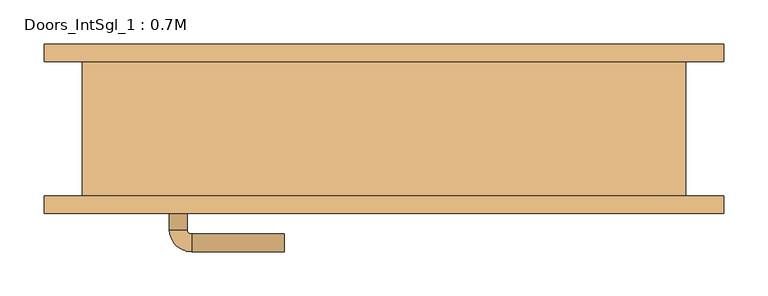
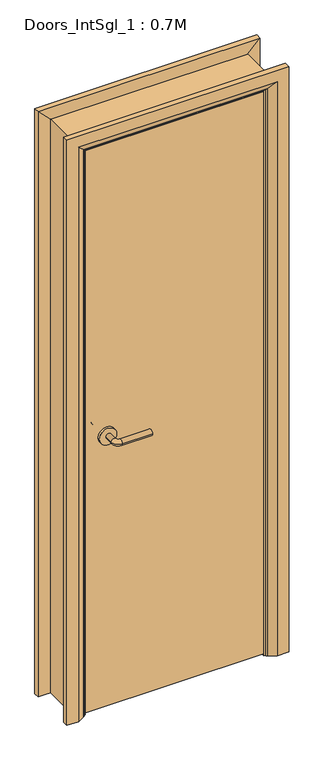
"""IFC4 building model written with IfcOpenShell, lengths in millimetres: door geometry, Doors_IntSgl_1 : 0.7M."""

from ifc_helpers import new_model, si_unit, point, frame, frame_2d, origin, place, context, project, spatial, polyline, circle_curve, ellipse_curve, trimmed, segment, composite_curve, outline, extrude, faceted_brep, source, transform, mapped, element, save
from ifc_brep_helpers import plane_surface, cylinder_surface, revolved_surface, advanced_brep


def doors_intsgl_1_0_7m_20e7f540(model_context):
    return source(origin(), model_context, "Body", "SolidModel", [
        advanced_brep(
        [(-243.0, -30.2, 1000.0), (-223.0, -30.2, 1000.0), (-243.0, -0.2, 1000.0), (-223.0, -0.2, 1000.0), (-218.0, 4.8, 1000.0), (-218.0, 24.8, 1000.0), (-113.0, 24.8, 1000.0), (-113.0, 4.8, 1000.0)],
        [
            (0, 1, circle_curve(frame((-233.0, -30.2, 1000.0), z_axis=(0.0, -1.0, 0.0), x_axis=(1.0, 0.0, 0.0)), 10.0)),
            (1, 0, circle_curve(frame((-233.0, -30.2, 1000.0), z_axis=(0.0, -1.0, 0.0), x_axis=(1.0, 0.0, 0.0)), 10.0)),
            (0, 2),
            (2, 3, circle_curve(frame((-233.0, -0.2, 1000.0), z_axis=(0.0, -1.0, 0.0), x_axis=(1.0, 0.0, 0.0)), 10.0)),
            (3, 1),
            (3, 2, circle_curve(frame((-233.0, -0.2, 1000.0), z_axis=(0.0, -1.0, 0.0), x_axis=(1.0, 0.0, 0.0)), 10.0)),
            (4, 3, circle_curve(frame((-218.0, -0.2, 1000.0), z_axis=(0.0, 0.0, 1.0), x_axis=(-1.0, 0.0, 0.0)), 5.0)),
            (2, 5, circle_curve(frame((-218.0, -0.2, 1000.0), z_axis=(0.0, 0.0, -1.0), x_axis=(-1.0, 0.0, 0.0)), 25.0)),
            (5, 4, circle_curve(frame((-218.0, 14.8, 1000.0), z_axis=(-1.0, 0.0, 0.0), x_axis=(0.0, -1.0, 0.0)), 10.0)),
            (4, 5, circle_curve(frame((-218.0, 14.8, 1000.0), z_axis=(-1.0, 0.0, 0.0), x_axis=(0.0, -1.0, 0.0)), 10.0)),
            (6, 7, circle_curve(frame((-113.0, 14.8, 1000.0), z_axis=(1.0, 0.0, 0.0), x_axis=(0.0, -1.0, 0.0)), 10.0)),
            (7, 6, circle_curve(frame((-113.0, 14.8, 1000.0), z_axis=(1.0, 0.0, 0.0), x_axis=(0.0, -1.0, 0.0)), 10.0)),
            (5, 6),
            (7, 4),
        ],
        [
            plane_surface(frame((-233.0, -30.2, 1000.0), z_axis=(0.0, -1.0, 0.0), x_axis=(0.0, 0.0, 1.0))),
            cylinder_surface(frame((-233.0, -30.2, 1000.0), z_axis=(0.0, -1.0, 0.0), x_axis=(1.0, 0.0, 0.0)), 10.0),
            revolved_surface(trimmed(ellipse_curve(frame((-233.0, -0.2, 1000.0), z_axis=(0.0, -1.0, 0.0), x_axis=(1.0, 0.0, 0.0)), 10.0, 10.0), [point((-243.0, -0.2, 1000.0))], [point((-223.0, -0.2, 1000.0))], True, "CARTESIAN"), (-218.0, -0.2, 1000.0), (0.0, 0.0, -1.0)),
            revolved_surface(trimmed(ellipse_curve(frame((-233.0, -0.2, 1000.0), z_axis=(0.0, -1.0, 0.0), x_axis=(1.0, 0.0, 0.0)), 10.0, 10.0), [point((-223.0, -0.2, 1000.0))], [point((-243.0, -0.2, 1000.0))], True, "CARTESIAN"), (-218.0, -0.2, 1000.0), (0.0, 0.0, -1.0)),
            plane_surface(frame((-113.0, 14.8, 1000.0), z_axis=(1.0, 0.0, 0.0), x_axis=(0.0, 0.0, 1.0))),
            cylinder_surface(frame((-218.0, 14.8, 1000.0), z_axis=(-1.0, 0.0, 0.0), x_axis=(0.0, -1.0, 0.0)), 10.0),
        ],
        [
            (0, [[1, 2]]),
            (1, [[-1, 3, 4, 5]]),
            (1, [[-2, -5, 6, -3]]),
            (2, [[7, -4, 8, 9]]),
            (3, [[-8, -6, -7, 10]]),
            (4, [[11, 12]]),
            (5, [[-9, 13, -12, 14]]),
            (5, [[-10, -14, -11, -13]]),
        ],
    ),
        extrude(outline(composite_curve([segment(trimmed(circle_curve(frame_2d((1000.0, -235.5)), 30.0), [point((1000.0, -265.5))], [point((1000.0, -205.5))], False, "CARTESIAN"), True, "CONTINUOUS"), segment(trimmed(circle_curve(frame_2d((1000.0, -235.5)), 30.0), [point((1000.0, -205.5))], [point((1000.0, -265.5))], False, "CARTESIAN"), True, "CONTINUOUS")], self_intersect=False)), frame((0.0, -38.2, 0.0), z_axis=(0.0, 1.0, 0.0), x_axis=(0.0, 0.0, 1.0)), (0.0, 0.0, 1.0), 8.0),
        advanced_brep(
        [(-243.0, -84.2, 1000.0), (-223.0, -84.2, 1000.0), (-223.0, -114.2, 1000.0), (-243.0, -114.2, 1000.0), (-218.0, -119.2, 1000.0), (-218.0, -139.2, 1000.0), (-113.0, -139.2, 1000.0), (-113.0, -119.2, 1000.0)],
        [
            (0, 1, circle_curve(frame((-233.0, -84.2, 1000.0), z_axis=(0.0, 1.0, 0.0), x_axis=(1.0, 0.0, 0.0)), 10.0)),
            (1, 0, circle_curve(frame((-233.0, -84.2, 1000.0), z_axis=(0.0, 1.0, 0.0), x_axis=(1.0, 0.0, 0.0)), 10.0)),
            (1, 2),
            (2, 3, circle_curve(frame((-233.0, -114.2, 1000.0), z_axis=(0.0, 1.0, 0.0), x_axis=(1.0, 0.0, 0.0)), 10.0)),
            (3, 0),
            (3, 2, circle_curve(frame((-233.0, -114.2, 1000.0), z_axis=(0.0, 1.0, 0.0), x_axis=(1.0, 0.0, 0.0)), 10.0)),
            (4, 5, circle_curve(frame((-218.0, -129.2, 1000.0), z_axis=(-1.0, 0.0, 0.0), x_axis=(0.0, 1.0, 0.0)), 10.0)),
            (5, 3, circle_curve(frame((-218.0, -114.2, 1000.0), z_axis=(0.0, 0.0, -1.0), x_axis=(-1.0, 0.0, 0.0)), 25.0)),
            (2, 4, circle_curve(frame((-218.0, -114.2, 1000.0), z_axis=(0.0, 0.0, 1.0), x_axis=(-1.0, 0.0, 0.0)), 5.0)),
            (5, 4, circle_curve(frame((-218.0, -129.2, 1000.0), z_axis=(-1.0, 0.0, 0.0), x_axis=(0.0, 1.0, 0.0)), 10.0)),
            (6, 7, circle_curve(frame((-113.0, -129.2, 1000.0), z_axis=(1.0, 0.0, 0.0), x_axis=(0.0, 1.0, 0.0)), 10.0)),
            (7, 6, circle_curve(frame((-113.0, -129.2, 1000.0), z_axis=(1.0, 0.0, 0.0), x_axis=(0.0, 1.0, 0.0)), 10.0)),
            (4, 7),
            (6, 5),
        ],
        [
            plane_surface(frame((-233.0, -84.2, 1000.0), z_axis=(0.0, 1.0, 0.0), x_axis=(0.0, 0.0, 1.0))),
            cylinder_surface(frame((-233.0, -84.2, 1000.0), z_axis=(0.0, 1.0, 0.0), x_axis=(1.0, 0.0, 0.0)), 10.0),
            revolved_surface(trimmed(ellipse_curve(frame((-233.0, -114.2, 1000.0), z_axis=(0.0, -1.0, 0.0), x_axis=(1.0, 0.0, 0.0)), 10.0, 10.0), [point((-243.0, -114.2, 1000.0))], [point((-223.0, -114.2, 1000.0))], True, "CARTESIAN"), (-218.0, -114.2, 1000.0), (0.0, 0.0, -1.0)),
            revolved_surface(trimmed(ellipse_curve(frame((-233.0, -114.2, 1000.0), z_axis=(0.0, -1.0, 0.0), x_axis=(1.0, 0.0, 0.0)), 10.0, 10.0), [point((-223.0, -114.2, 1000.0))], [point((-243.0, -114.2, 1000.0))], True, "CARTESIAN"), (-218.0, -114.2, 1000.0), (0.0, 0.0, -1.0)),
            plane_surface(frame((-113.0, -129.2, 1000.0), z_axis=(1.0, 0.0, 0.0), x_axis=(0.0, 0.0, 1.0))),
            cylinder_surface(frame((-218.0, -129.2, 1000.0), z_axis=(-1.0, 0.0, 0.0), x_axis=(0.0, 1.0, 0.0)), 10.0),
        ],
        [
            (0, [[1, 2]]),
            (1, [[3, 4, 5, -2]]),
            (1, [[-5, 6, -3, -1]]),
            (2, [[7, 8, -4, 9]]),
            (3, [[10, -9, -6, -8]]),
            (4, [[11, 12]]),
            (5, [[13, -11, 14, -7]]),
            (5, [[-14, -12, -13, -10]]),
        ],
    ),
        extrude(outline(composite_curve([segment(trimmed(circle_curve(frame_2d((1000.0, -235.5)), 30.0), [point((1000.0, -265.5))], [point((1000.0, -205.5))], False, "CARTESIAN"), True, "CONTINUOUS"), segment(trimmed(circle_curve(frame_2d((1000.0, -235.5)), 30.0), [point((1000.0, -205.5))], [point((1000.0, -265.5))], False, "CARTESIAN"), True, "CONTINUOUS")], self_intersect=False)), frame((0.0, -84.2, 0.0), z_axis=(0.0, 1.0, 0.0), x_axis=(0.0, 0.0, 1.0)), (0.0, 0.0, 1.0), 8.0),
        extrude(outline(polyline([(308.0, -38.2), (308.0, -76.2), (-308.0, -76.2), (-308.0, -38.2), (308.0, -38.2)])), frame((0.0, 0.0, 8.0), z_axis=(0.0, 0.0, 1.0), x_axis=(1.0, 0.0, 0.0)), (0.0, 0.0, 1.0), 2060.0),
        faceted_brep([(-310.0, -76.2, 0.0), (-342.0, -76.2, 0.0), (-342.0, 76.2, 0.0), (-310.0, 76.2, 0.0), (-310.0, 76.2, 2070.0), (-310.0, -76.2, 2070.0), (-342.0, 76.2, 2102.0), (-342.0, -76.2, 2102.0), (310.0, -76.2, 0.0), (310.0, 76.2, 0.0), (342.0, 76.2, 0.0), (342.0, -76.2, 0.0), (310.0, -76.2, 2070.0), (342.0, -76.2, 2102.0), (342.0, 76.2, 2102.0), (310.0, 76.2, 2070.0)], [[[0, 1, 2, 3]], [[3, 4, 5, 0]], [[2, 6, 4, 3]], [[1, 7, 6, 2]], [[0, 5, 7, 1]], [[8, 9, 10, 11]], [[12, 8, 11, 13]], [[13, 11, 10, 14]], [[14, 10, 9, 15]], [[15, 9, 8, 12]], [[4, 15, 12, 5]], [[6, 14, 15, 4]], [[7, 13, 14, 6]], [[5, 12, 13, 7]]]),
        advanced_brep(
        [(-385.0, 96.2, 0.0), (-345.0, 96.2, 0.0), (-319.0, 82.2, 0.0), (-315.0, 76.2, 0.0), (-385.0, 76.2, 0.0), (-385.0, 76.2, 2145.0), (-385.0, 96.2, 2145.0), (-315.0, 76.2, 2075.0), (-319.0, 82.2, 2079.0), (-345.0, 96.2, 2105.0), (385.0, 96.2, 0.0), (385.0, 76.2, 0.0), (315.0, 76.2, 0.0), (319.0, 82.2, 0.0), (345.0, 96.2, 0.0), (385.0, 96.2, 2145.0), (345.0, 96.2, 2105.0), (319.0, 82.2, 2079.0), (315.0, 76.2, 2075.0), (385.0, 76.2, 2145.0)],
        [
            (0, 1),
            (1, 2),
            (2, 3, circle_curve(frame((-323.0, 75.2, 0.0), z_axis=(0.0, 0.0, -1.0), x_axis=(-1.0, 0.0, 0.0)), 8.0622577)),
            (3, 4),
            (4, 0),
            (4, 5),
            (5, 6),
            (6, 0),
            (3, 7),
            (7, 5),
            (2, 8),
            (8, 7, ellipse_curve(frame((-323.0, 75.2, 2083.0), z_axis=(-0.7071067811865475, 0.0, -0.7071067811865475), x_axis=(0.7071067811865474, 0.0, -0.7071067811865476)), 11.4017543, 8.0622577)),
            (1, 9),
            (9, 8),
            (6, 9),
            (10, 11),
            (11, 12),
            (12, 13, circle_curve(frame((323.0, 75.2, 0.0), z_axis=(0.0, 0.0, -1.0), x_axis=(1.0, 0.0, 0.0)), 8.0622577)),
            (13, 14),
            (14, 10),
            (15, 10),
            (14, 16),
            (16, 15),
            (13, 17),
            (17, 16),
            (12, 18),
            (18, 17, ellipse_curve(frame((323.0, 75.2, 2083.0), z_axis=(0.7071067811865475, 0.0, -0.7071067811865475), x_axis=(0.7071067811865474, 0.0, 0.7071067811865476)), 11.4017543, 8.0622577)),
            (11, 19),
            (19, 18),
            (15, 19),
            (5, 19),
            (15, 6),
            (7, 18),
            (8, 17),
            (9, 16),
        ],
        [
            plane_surface(frame((-315.0, 149.0010989, 0.0), z_axis=(0.0, 0.0, -1.0), x_axis=(1.0, 0.0, 0.0))),
            plane_surface(frame((-385.0, 96.2, 0.0), z_axis=(-1.0, 0.0, 0.0), x_axis=(0.0, 0.0, 1.0))),
            plane_surface(frame((-385.0, 76.2, 0.0), z_axis=(0.0, -1.0, 0.0), x_axis=(0.0, 0.0, 1.0))),
            cylinder_surface(frame((-323.0, 75.2, 0.0), z_axis=(0.0, 0.0, -1.0), x_axis=(-1.0, 0.0, 0.0)), 8.0622577),
            plane_surface(frame((-319.0, 82.2, 0.0), z_axis=(0.4740998230350183, 0.8804710999221749, 0.0), x_axis=(0.0, 0.0, 1.0))),
            plane_surface(frame((-345.0, 96.2, 0.0), z_axis=(0.0, 1.0, 0.0), x_axis=(0.0, 0.0, 1.0))),
            plane_surface(frame((315.0, 149.0010989, 0.0), z_axis=(0.0, 0.0, -1.0), x_axis=(-1.0, 0.0, 0.0))),
            plane_surface(frame((345.0, 96.2, 2105.0), z_axis=(0.0, 1.0, 0.0), x_axis=(0.0, 0.0, -1.0))),
            plane_surface(frame((319.0, 82.2, 2079.0), z_axis=(-0.4740998230350183, 0.8804710999221749, 0.0), x_axis=(0.0, 0.0, -1.0))),
            cylinder_surface(frame((323.0, 75.2, 2075.0), z_axis=(0.0, 0.0, 1.0), x_axis=(1.0, 0.0, 0.0)), 8.0622577),
            plane_surface(frame((385.0, 76.2, 2145.0), z_axis=(0.0, -1.0, 0.0), x_axis=(0.0, 0.0, -1.0))),
            plane_surface(frame((385.0, 96.2, 2145.0), z_axis=(1.0, 0.0, 0.0), x_axis=(0.0, 0.0, -1.0))),
            plane_surface(frame((-385.0, 96.2, 2145.0), z_axis=(0.0, 0.0, 1.0), x_axis=(1.0, 0.0, 0.0))),
            plane_surface(frame((-385.0, 76.2, 2145.0), z_axis=(0.0, -1.0, 0.0), x_axis=(1.0, 0.0, 0.0))),
            cylinder_surface(frame((-315.0, 75.2, 2083.0), z_axis=(-1.0, 0.0, 0.0), x_axis=(0.0, 0.0, 1.0)), 8.0622577),
            plane_surface(frame((-319.0, 82.2, 2079.0), z_axis=(0.0, 0.8804710999221749, -0.4740998230350183), x_axis=(1.0, 0.0, 0.0))),
            plane_surface(frame((-345.0, 96.2, 2105.0), z_axis=(0.0, 1.0, 0.0), x_axis=(1.0, 0.0, 0.0))),
        ],
        [
            (0, [[1, 2, 3, 4, 5]]),
            (1, [[6, 7, 8, -5]]),
            (2, [[9, 10, -6, -4]]),
            (3, [[11, 12, -9, -3]]),
            (4, [[13, 14, -11, -2]]),
            (5, [[-8, 15, -13, -1]]),
            (6, [[16, 17, 18, 19, 20]]),
            (7, [[21, -20, 22, 23]]),
            (8, [[-22, -19, 24, 25]]),
            (9, [[-24, -18, 26, 27]]),
            (10, [[-26, -17, 28, 29]]),
            (11, [[-28, -16, -21, 30]]),
            (12, [[31, -30, 32, -7]]),
            (13, [[33, -29, -31, -10]]),
            (14, [[34, -27, -33, -12]]),
            (15, [[35, -25, -34, -14]]),
            (16, [[-32, -23, -35, -15]]),
        ],
    ),
        extrude(outline(polyline([(0.0, -291.0), (2051.0, -291.0), (2051.0, 291.0), (0.0, 291.0), (0.0, 310.0), (2070.0, 310.0), (2070.0, -310.0), (0.0, -310.0), (0.0, -291.0)])), frame((0.0, -36.2, 0.0), z_axis=(0.0, 1.0, 0.0), x_axis=(0.0, 0.0, 1.0)), (0.0, 0.0, 1.0), 32.0),
        advanced_brep(
        [(385.0, -96.2, 0.0), (345.0, -96.2, 0.0), (319.0, -82.2, 0.0), (315.0, -76.2, 0.0), (385.0, -76.2, 0.0), (385.0, -76.2, 2145.0), (385.0, -96.2, 2145.0), (315.0, -76.2, 2075.0), (-315.0, -76.2, 2075.0), (-315.0, -76.2, 0.0), (-385.0, -76.2, 0.0), (-385.0, -76.2, 2145.0), (319.0, -82.2, 2079.0), (345.0, -96.2, 2105.0), (-385.0, -96.2, 2145.0), (-385.0, -96.2, 0.0), (-345.0, -96.2, 0.0), (-345.0, -96.2, 2105.0), (-319.0, -82.2, 0.0), (-319.0, -82.2, 2079.0)],
        [
            (0, 1),
            (1, 2),
            (2, 3, circle_curve(frame((323.0, -75.2, 0.0), z_axis=(0.0, 0.0, -1.0), x_axis=(1.0, 0.0, 0.0)), 8.0622577)),
            (3, 4),
            (4, 0),
            (4, 5),
            (5, 6),
            (6, 0),
            (3, 7),
            (7, 8),
            (8, 9),
            (9, 10),
            (10, 11),
            (11, 5),
            (2, 12),
            (12, 7, ellipse_curve(frame((323.0, -75.2, 2083.0), z_axis=(0.7071067811865475, 0.0, -0.7071067811865475), x_axis=(-0.7071067811865474, 0.0, -0.7071067811865476)), 11.4017543, 8.0622577)),
            (1, 13),
            (13, 12),
            (6, 14),
            (14, 15),
            (15, 16),
            (16, 17),
            (17, 13),
            (10, 15),
            (14, 11),
            (9, 18, circle_curve(frame((-323.0, -75.2, 0.0), z_axis=(0.0, 0.0, -1.0), x_axis=(-1.0, 0.0, 0.0)), 8.0622577)),
            (18, 16),
            (19, 18),
            (8, 19, ellipse_curve(frame((-323.0, -75.2, 2083.0), z_axis=(-0.7071067811865475, 0.0, -0.7071067811865475), x_axis=(-0.7071067811865474, 0.0, 0.7071067811865476)), 11.4017543, 8.0622577)),
            (19, 17),
            (12, 19),
        ],
        [
            plane_surface(frame((315.0, -76.2, 0.0), z_axis=(0.0, 0.0, -1.0), x_axis=(0.0, 1.0, 0.0))),
            plane_surface(frame((385.0, -96.2, 0.0), z_axis=(1.0, 0.0, 0.0), x_axis=(0.0, 0.0, 1.0))),
            plane_surface(frame((385.0, -76.2, 0.0), z_axis=(0.0, 1.0, 0.0), x_axis=(0.0, 0.0, 1.0))),
            cylinder_surface(frame((323.0, -75.2, 0.0), z_axis=(0.0, 0.0, -1.0), x_axis=(1.0, 0.0, 0.0)), 8.0622577),
            plane_surface(frame((319.0, -82.2, 0.0), z_axis=(-0.4740998230350126, -0.880471099922178, 0.0), x_axis=(0.0, 0.0, 1.0))),
            plane_surface(frame((345.0, -96.2, 0.0), z_axis=(0.0, -1.0, 0.0), x_axis=(0.0, 0.0, 1.0))),
            plane_surface(frame((-385.0, -96.2, 2145.0), z_axis=(-1.0, 0.0, 0.0), x_axis=(0.0, 0.0, -1.0))),
            plane_surface(frame((-315.0, -76.2, 0.0), z_axis=(0.0, 0.0, -1.0), x_axis=(0.0, 1.0, 0.0))),
            cylinder_surface(frame((-323.0, -75.2, 2075.0), z_axis=(0.0, 0.0, 1.0), x_axis=(-1.0, 0.0, 0.0)), 8.0622577),
            plane_surface(frame((-319.0, -82.2, 2079.0), z_axis=(0.47409982303501824, -0.8804710999221749, 0.0), x_axis=(0.0, 0.0, -1.0))),
            plane_surface(frame((385.0, -96.2, 2145.0), z_axis=(0.0, 0.0, 1.0), x_axis=(-1.0, 0.0, 0.0))),
            cylinder_surface(frame((315.0, -75.2, 2083.0), z_axis=(1.0, 0.0, 0.0), x_axis=(0.0, 0.0, 1.0)), 8.0622577),
            plane_surface(frame((319.0, -82.2, 2079.0), z_axis=(0.0, -0.8804710999221764, -0.4740998230350154), x_axis=(-1.0, 0.0, 0.0))),
        ],
        [
            (0, [[1, 2, 3, 4, 5]]),
            (1, [[6, 7, 8, -5]]),
            (2, [[9, 10, 11, 12, 13, 14, -6, -4]]),
            (3, [[15, 16, -9, -3]]),
            (4, [[17, 18, -15, -2]]),
            (5, [[-8, 19, 20, 21, 22, 23, -17, -1]]),
            (6, [[-13, 24, -20, 25]]),
            (7, [[-24, -12, 26, 27, -21]]),
            (8, [[28, -26, -11, 29]]),
            (9, [[-22, -27, -28, 30]]),
            (10, [[-14, -25, -19, -7]]),
            (11, [[31, -29, -10, -16]]),
            (12, [[-23, -30, -31, -18]]),
        ],
    ),
    ])


if __name__ == "__main__":
    model = new_model("IFC4")
    model_context = context("Model", 3, world=origin())
    ifc_project = project(units=[si_unit("LENGTHUNIT", "METRE", prefix="MILLI")], contexts=[model_context])
    site = spatial("IfcSite", under=ifc_project)
    building = spatial("IfcBuilding", under=site)
    placement = place(None, origin())
    doors_intsgl_1_0_7m_shape = doors_intsgl_1_0_7m_20e7f540(model_context)
    element("IfcDoor", 1, ObjectType="Doors_IntSgl_1 : 0.7M", at=placement, inside=building, context=model_context, shape_type="MappedRepresentation", body=[
        mapped(doors_intsgl_1_0_7m_shape, transform((0.0, 0.0, 0.0), x_axis=(1.0, 0.0, 0.0), y_axis=(0.0, 1.0, 0.0), z_axis=(0.0, 0.0, 1.0))),
    ])
    save(model, "model.ifc")

# Revit data of these elements
# Type "Doors_IntSgl_1 : 0.7M"
#   Type Mark = "58"
#   Type Comments = "Internal Single"
#   Operation = "SingleSwingRight"
#   Construction Type Id = "MDOOR"
#   Manufacturer = "Revit"
#   Keynote = "L20"
#   Description = "Internal Single Door"
#   Analytic Construction = "Metal"
#   UnderCut = 0.008 m
#   Tolerance = 0.002 m
#   Thickness = 0.038 m
#   Structural Tolerance = 0.008 m
#   StopDepth = 0.032 m
#   Stop Thickness = 0.019 m
#   Rough Width = 0.7 m
#   Rough Height = 2.11 m
#   Height to Top Lock Rail = 1.0 m
#   Heat Transfer Coefficient (U) = 3.7021 W/(m²·K)
#   Handle Z Distance = 1.0 m
#   Handle X Distance = 0.075 m
#   Frame Thickness = 0.032 m
#   Door Panel Width = 0.616 m
#   Door Panel Thickness = 0.038 m
#   Door Panel Offset = 0.0 m
#   Height = 2.11 m
#   Width = 0.7 m
#   Door Panel Height = 2.06 m
#   Architrave Setback = 0.005 m
#   Vis - Ironmongery = yes
#   Define Thermal Properties by = 1
#   Material Ironmongery = Door - Handle
#   Material Frame = Door - Frame/Mullion
#   Material Door = Door - Panel
#   Material Architrave = Door - Architrave
#   Visual Light Transmittance = 0
#   Solar Heat Gain Coefficient = 0
#   Function = (empty or 0)
#   Wall Closure = (empty or 0)
# Element 1 (IfcDoor, "Doors_IntSgl_1 : 0.7M")
#   Materials on its faces: "Door - Architrave", "Door - Handle", "Door - Frame/Mullion", "Door - Panel"
# Materials
#   "Door - Handle": colour RGB 0 0 0, transparency 0, Keynote = "P21", Cost = 0
#   "Door - Frame/Mullion": class "Wood", colour RGB 212 179 113, transparency 0, Keynote = "L20", Cost = 0
#   "Door - Panel": class "Wood", colour RGB 210 159 95, transparency 0, Keynote = "L20", Cost = 0
#   "Door - Architrave": class "Wood", colour RGB 154 90 5, transparency 0, Keynote = "P20", Cost = 0
